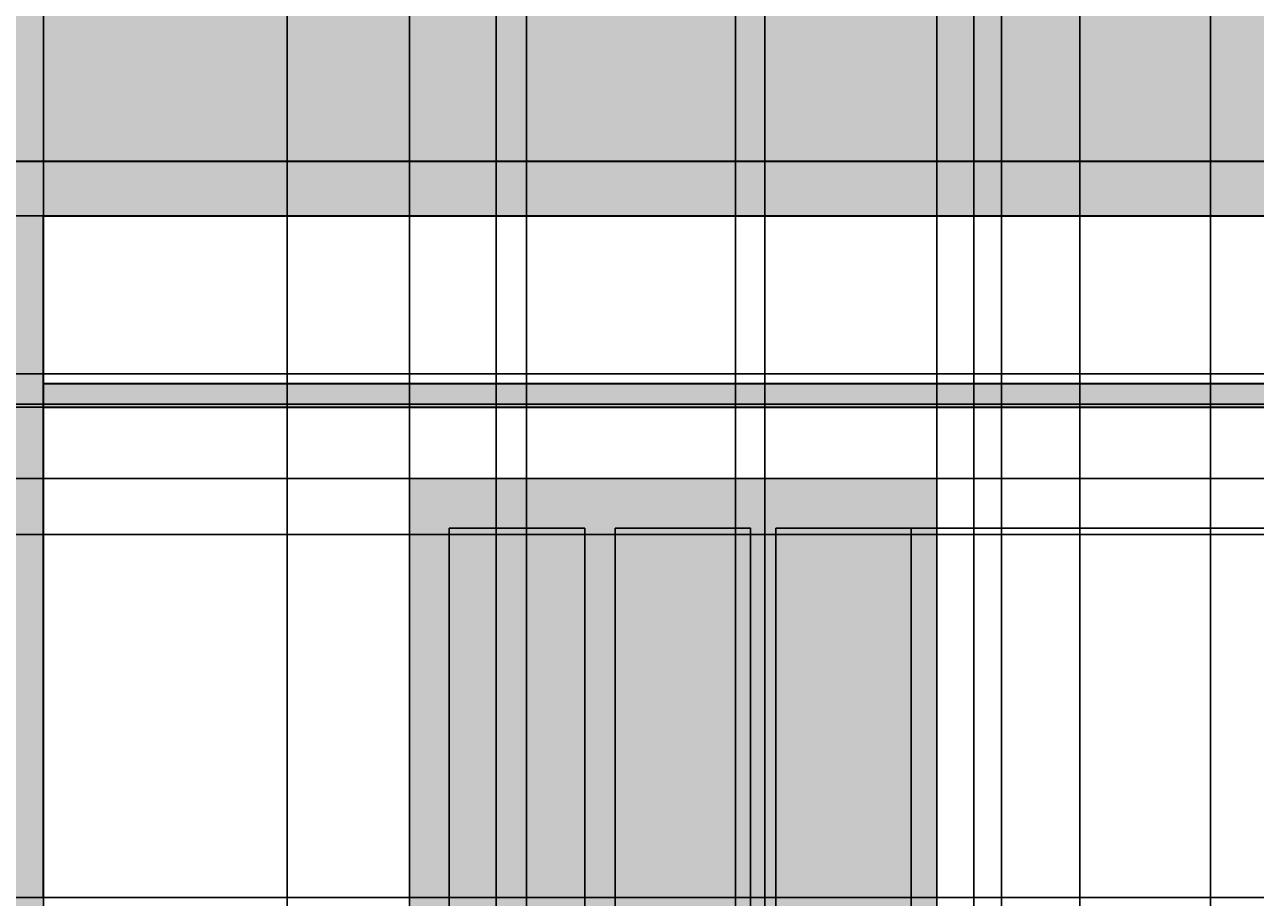
# Model space of a CAD drawing. Units: inches. Extents: x -5 to 714, y 84 to 644.
# Tile 6 of 20: x 266 to 457, y 201 to 336. Entities that reach past the tile are written whole.
import ezdxf

# ---------------------------------------------------------------- set-up
doc = ezdxf.new("R2010")
doc.units = ezdxf.units.IN
doc.header["$MEASUREMENT"] = 0
for name, color, linetype, lineweight in [('A-ANNO-DIMS', 2, 'Continuous', 18), ('A-ELEV', 7, 'Continuous', 35), ('A-ELEV-PATT', 8, 'Continuous', 13), ('A-GLAZ', 3, 'Continuous', 25)]:
    doc.layers.add(name, color=color, linetype=linetype, lineweight=lineweight)
doc.styles.get("Standard").update_dxf_attribs({"font": 'arial.ttf'})
doc.dimstyles.get("Standard").update_dxf_attribs({"dimtxt": 0.9375, "dimasz": 0.18, "dimexe": 0.18, "dimexo": 0.0625, "dimgap": 0.09, "dimtad": 0, "dimtih": 1, "dimtoh": 1, "dimdec": 4, "dimzin": 0, "dimdsep": 46, "dimlunit": 4, "dimtxsty": 'Standard', "dimcen": 0.09, "dimadec": 0, "dimazin": 0, "dimtfac": 1, "dimtdec": 4, "dimtofl": 0, "dimtmove": 0, "dimatfit": 3, "dimfxl": 1, "dimtolj": 1, "dimtzin": 0, "dimarcsym": 0})

# ---------------------------------------------------------------- blocks, each defined once
blk = doc.blocks.new('*D29')
at = {"layer": 'A-ANNO-DIMS', "color": 0, "lineweight": -2, "transparency": 16777216}
for p, q in [((135.73, 471.11), (135.73, 84.31)), ((429.51, 471.11), (429.51, 84.31)), ((135.91, 84.49), (280.94, 84.49)), ((429.33, 84.49), (284.3, 84.49))]:
    blk.add_line(p, q, dxfattribs=at)
at = {"layer": 'A-ANNO-DIMS', "color": 0, "transparency": 16777216}
for points in [[(135.91, 84.52), (135.91, 84.46), (135.73, 84.49)], [(429.33, 84.52), (429.33, 84.46), (429.51, 84.49)]]:
    blk.add_solid(points, dxfattribs=at)
at = {"layer": 'Defpoints', "color": 0, "transparency": 16777216}
for p in [(135.73, 471.17), (429.51, 471.17), (429.51, 84.49)]:
    blk.add_point(p, dxfattribs=at)
at = {"layer": 'A-ANNO-DIMS', "color": 0, "transparency": 16777216, "insert": (282.62, 84.49), "char_height": 0.938, "attachment_point": 5}
blk.add_mtext('\\A1;293.8', dxfattribs=at)
blk = doc.blocks.new('*D53')
at = {"layer": 'A-ANNO-DIMS', "color": 0, "lineweight": -2, "transparency": 16777216}
for p, q in [((259.07, 315.03), (259.07, 84.31)), ((269.24, 306.57), (269.24, 84.31)), ((259.25, 84.49), (262.16, 84.49)), ((269.06, 84.49), (266.15, 84.49))]:
    blk.add_line(p, q, dxfattribs=at)
at = {"layer": 'A-ANNO-DIMS', "color": 0, "transparency": 16777216}
for points in [[(259.25, 84.52), (259.25, 84.46), (259.07, 84.49)], [(269.06, 84.52), (269.06, 84.46), (269.24, 84.49)]]:
    blk.add_solid(points, dxfattribs=at)
at = {"layer": 'Defpoints', "color": 0, "transparency": 16777216}
for p in [(259.07, 315.1), (269.24, 306.63), (269.24, 84.49)]:
    blk.add_point(p, dxfattribs=at)
at = {"layer": 'A-ANNO-DIMS', "color": 0, "transparency": 16777216, "insert": (264.16, 84.49), "char_height": 0.938, "attachment_point": 5}
blk.add_mtext('\\A1;10.178', dxfattribs=at)
blk = doc.blocks.new('*D54')
at = {"layer": 'A-ANNO-DIMS', "color": 0, "lineweight": -2, "transparency": 16777216}
for p, q in [((259.07, 315.16), (259.07, 643.61)), ((259.25, 643.43), (424.21, 643.43)), ((593.25, 643.43), (428.28, 643.43)), ((593.43, 315.16), (593.43, 643.61))]:
    blk.add_line(p, q, dxfattribs=at)
at = {"layer": 'A-ANNO-DIMS', "color": 0, "transparency": 16777216}
for points in [[(259.25, 643.46), (259.25, 643.4), (259.07, 643.43)], [(593.25, 643.46), (593.25, 643.4), (593.43, 643.43)]]:
    blk.add_solid(points, dxfattribs=at)
at = {"layer": 'Defpoints', "color": 0, "transparency": 16777216}
for p in [(593.43, 643.43), (259.07, 315.1), (593.43, 315.1)]:
    blk.add_point(p, dxfattribs=at)
at = {"layer": 'A-ANNO-DIMS', "color": 0, "transparency": 16777216, "insert": (426.25, 643.43), "char_height": 0.938, "attachment_point": 5}
blk.add_mtext('\\A1;334.36', dxfattribs=at)
blk = doc.blocks.new('*D56')
at = {"layer": 'A-ANNO-DIMS', "color": 0, "lineweight": -2, "transparency": 16777216}
for p, q in [((578.03, 277.05), (-2.74, 277.05)), ((-2.56, 276.87), (-2.56, 239.69)), ((-2.56, 201.37), (-2.56, 238.55)), ((578.03, 201.19), (-2.74, 201.19))]:
    blk.add_line(p, q, dxfattribs=at)
at = {"layer": 'A-ANNO-DIMS', "color": 0, "transparency": 16777216}
for points in [[(-2.59, 276.87), (-2.53, 276.87), (-2.56, 277.05)], [(-2.59, 201.37), (-2.53, 201.37), (-2.56, 201.19)]]:
    blk.add_solid(points, dxfattribs=at)
at = {"layer": 'Defpoints', "color": 0, "transparency": 16777216}
for p in [(-2.56, 277.05), (578.09, 277.05), (578.09, 201.19)]:
    blk.add_point(p, dxfattribs=at)
at = {"layer": 'A-ANNO-DIMS', "color": 0, "transparency": 16777216, "insert": (-2.56, 239.12), "char_height": 0.938, "attachment_point": 5}
blk.add_mtext('\\A1;75.86', dxfattribs=at)
blk = doc.blocks.new('*D57')
at = {"layer": 'A-ANNO-DIMS', "color": 0, "lineweight": -2, "transparency": 16777216}
for p, q in [((578.03, 306.63), (-2.74, 306.63)), ((-2.56, 306.45), (-2.56, 292.41)), ((-2.56, 277.23), (-2.56, 291.27)), ((578.03, 277.05), (-2.74, 277.05))]:
    blk.add_line(p, q, dxfattribs=at)
at = {"layer": 'A-ANNO-DIMS', "color": 0, "transparency": 16777216}
for points in [[(-2.59, 306.45), (-2.53, 306.45), (-2.56, 306.63)], [(-2.59, 277.23), (-2.53, 277.23), (-2.56, 277.05)]]:
    blk.add_solid(points, dxfattribs=at)
at = {"layer": 'Defpoints', "color": 0, "transparency": 16777216}
for p in [(578.09, 306.63), (-2.56, 277.05), (578.09, 277.05)]:
    blk.add_point(p, dxfattribs=at)
at = {"layer": 'A-ANNO-DIMS', "color": 0, "transparency": 16777216, "insert": (-2.56, 291.84), "char_height": 0.938, "attachment_point": 5}
blk.add_mtext('\\A1;29.58', dxfattribs=at)
blk = doc.blocks.new('*D59')
at = {"layer": 'A-ANNO-DIMS', "color": 0, "lineweight": -2, "transparency": 16777216}
for p, q in [((593.37, 282.2), (-2.74, 282.2)), ((-2.56, 282.02), (-2.56, 280.41)), ((-2.56, 277.66), (-2.56, 279.27)), ((593.37, 277.48), (-2.74, 277.48))]:
    blk.add_line(p, q, dxfattribs=at)
at = {"layer": 'A-ANNO-DIMS', "color": 0, "transparency": 16777216}
for points in [[(-2.59, 282.02), (-2.53, 282.02), (-2.56, 282.2)], [(-2.59, 277.66), (-2.53, 277.66), (-2.56, 277.48)]]:
    blk.add_solid(points, dxfattribs=at)
at = {"layer": 'Defpoints', "color": 0, "transparency": 16777216}
for p in [(-2.56, 282.2), (593.43, 282.2), (593.43, 277.48)]:
    blk.add_point(p, dxfattribs=at)
at = {"layer": 'A-ANNO-DIMS', "color": 0, "transparency": 16777216, "insert": (-2.56, 279.84), "char_height": 0.938, "attachment_point": 5}
blk.add_mtext('\\A1;4.719', dxfattribs=at)
blk = doc.blocks.new('*D60')
at = {"layer": 'A-ANNO-DIMS', "color": 0, "lineweight": -2, "transparency": 16777216}
for p, q in [((269.24, 277.11), (269.24, 643.61)), ((269.42, 643.43), (295.86, 643.43)), ((325.65, 643.43), (299.21, 643.43)), ((325.83, 266.06), (325.83, 643.61))]:
    blk.add_line(p, q, dxfattribs=at)
at = {"layer": 'A-ANNO-DIMS', "color": 0, "transparency": 16777216}
for points in [[(269.42, 643.46), (269.42, 643.4), (269.24, 643.43)], [(325.65, 643.46), (325.65, 643.4), (325.83, 643.43)]]:
    blk.add_solid(points, dxfattribs=at)
at = {"layer": 'Defpoints', "color": 0, "transparency": 16777216}
for p in [(325.83, 643.43), (269.24, 277.05), (325.83, 266)]:
    blk.add_point(p, dxfattribs=at)
at = {"layer": 'A-ANNO-DIMS', "color": 0, "transparency": 16777216, "insert": (297.54, 643.43), "char_height": 0.938, "attachment_point": 5}
blk.add_mtext('\\A1;56.59', dxfattribs=at)
blk = doc.blocks.new('*D61')
at = {"layer": 'A-ANNO-DIMS', "color": 0, "lineweight": -2, "transparency": 16777216}
for p, q in [((325.83, 266.06), (325.83, 643.61)), ((326.01, 643.43), (364.93, 643.43)), ((407.2, 643.43), (368.28, 643.43)), ((407.38, 266.06), (407.38, 643.61))]:
    blk.add_line(p, q, dxfattribs=at)
at = {"layer": 'A-ANNO-DIMS', "color": 0, "transparency": 16777216}
for points in [[(326.01, 643.46), (326.01, 643.4), (325.83, 643.43)], [(407.2, 643.46), (407.2, 643.4), (407.38, 643.43)]]:
    blk.add_solid(points, dxfattribs=at)
at = {"layer": 'Defpoints', "color": 0, "transparency": 16777216}
for p in [(407.38, 643.43), (325.83, 266), (407.38, 266)]:
    blk.add_point(p, dxfattribs=at)
at = {"layer": 'A-ANNO-DIMS', "color": 0, "transparency": 16777216, "insert": (366.61, 643.43), "char_height": 0.938, "attachment_point": 5}
blk.add_mtext('\\A1;81.55', dxfattribs=at)
blk = doc.blocks.new('*D62')
at = {"layer": 'A-ANNO-DIMS', "color": 0, "lineweight": -2, "transparency": 16777216}
for p, q in [((407.38, 266.06), (407.38, 643.61)), ((407.56, 643.43), (449.27, 643.43)), ((493.6, 643.43), (451.89, 643.43)), ((493.78, 266.06), (493.78, 643.61))]:
    blk.add_line(p, q, dxfattribs=at)
at = {"layer": 'A-ANNO-DIMS', "color": 0, "transparency": 16777216}
for points in [[(407.56, 643.46), (407.56, 643.4), (407.38, 643.43)], [(493.6, 643.46), (493.6, 643.4), (493.78, 643.43)]]:
    blk.add_solid(points, dxfattribs=at)
at = {"layer": 'Defpoints', "color": 0, "transparency": 16777216}
for p in [(493.78, 643.43), (407.38, 266), (493.78, 266)]:
    blk.add_point(p, dxfattribs=at)
at = {"layer": 'A-ANNO-DIMS', "color": 0, "transparency": 16777216, "insert": (450.58, 643.43), "char_height": 0.938, "attachment_point": 5}
blk.add_mtext('\\A1;86.4', dxfattribs=at)
blk = doc.blocks.new('*D65')
at = {"layer": 'A-ANNO-DIMS', "color": 0, "lineweight": -2, "transparency": 16777216}
for p, q in [((325.77, 266), (-2.74, 266)), ((-2.56, 265.82), (-2.56, 219.13)), ((-2.56, 171.3), (-2.56, 217.99)), ((325.77, 171.12), (-2.74, 171.12))]:
    blk.add_line(p, q, dxfattribs=at)
at = {"layer": 'A-ANNO-DIMS', "color": 0, "transparency": 16777216}
for points in [[(-2.59, 265.82), (-2.53, 265.82), (-2.56, 266)], [(-2.59, 171.3), (-2.53, 171.3), (-2.56, 171.12)]]:
    blk.add_solid(points, dxfattribs=at)
at = {"layer": 'Defpoints', "color": 0, "transparency": 16777216}
for p in [(-2.56, 266), (325.83, 266), (325.83, 171.12)]:
    blk.add_point(p, dxfattribs=at)
at = {"layer": 'A-ANNO-DIMS', "color": 0, "transparency": 16777216, "insert": (-2.56, 218.56), "char_height": 0.938, "attachment_point": 5}
blk.add_mtext('\\A1;94.88', dxfattribs=at)
blk = doc.blocks.new('*D66')
at = {"layer": 'A-ANNO-DIMS', "color": 0, "lineweight": -2, "transparency": 16777216}
for p, q in [((332.01, 258.22), (332.01, 84.31)), ((352.95, 258.22), (352.95, 84.31)), ((332.19, 84.49), (340.43, 84.49)), ((352.77, 84.49), (344.52, 84.49))]:
    blk.add_line(p, q, dxfattribs=at)
at = {"layer": 'A-ANNO-DIMS', "color": 0, "transparency": 16777216}
for points in [[(332.19, 84.52), (332.19, 84.46), (332.01, 84.49)], [(352.77, 84.52), (352.77, 84.46), (352.95, 84.49)]]:
    blk.add_solid(points, dxfattribs=at)
at = {"layer": 'Defpoints', "color": 0, "transparency": 16777216}
for p in [(332.01, 258.29), (352.95, 258.29), (352.95, 84.49)]:
    blk.add_point(p, dxfattribs=at)
at = {"layer": 'A-ANNO-DIMS', "color": 0, "transparency": 16777216, "insert": (342.48, 84.49), "char_height": 0.938, "attachment_point": 5}
blk.add_mtext('\\A1;20.943', dxfattribs=at)
blk = doc.blocks.new('*D67')
at = {"layer": 'A-ANNO-DIMS', "color": 0, "lineweight": -2, "transparency": 16777216}
for p, q in [((357.65, 258.22), (357.65, 84.31)), ((378.6, 258.22), (378.6, 84.31)), ((357.83, 84.49), (366.08, 84.49)), ((378.42, 84.49), (370.17, 84.49))]:
    blk.add_line(p, q, dxfattribs=at)
at = {"layer": 'A-ANNO-DIMS', "color": 0, "transparency": 16777216}
for points in [[(357.83, 84.52), (357.83, 84.46), (357.65, 84.49)], [(378.42, 84.52), (378.42, 84.46), (378.6, 84.49)]]:
    blk.add_solid(points, dxfattribs=at)
at = {"layer": 'Defpoints', "color": 0, "transparency": 16777216}
for p in [(357.65, 258.29), (378.6, 258.29), (378.6, 84.49)]:
    blk.add_point(p, dxfattribs=at)
at = {"layer": 'A-ANNO-DIMS', "color": 0, "transparency": 16777216, "insert": (368.12, 84.49), "char_height": 0.938, "attachment_point": 5}
blk.add_mtext('\\A1;20.943', dxfattribs=at)
blk = doc.blocks.new('*D68')
at = {"layer": 'A-ANNO-DIMS', "color": 0, "lineweight": -2, "transparency": 16777216}
for p, q in [((382.5, 258.22), (382.5, 84.31)), ((403.44, 258.22), (403.44, 84.31)), ((382.68, 84.49), (390.92, 84.49)), ((403.26, 84.49), (395.01, 84.49))]:
    blk.add_line(p, q, dxfattribs=at)
at = {"layer": 'A-ANNO-DIMS', "color": 0, "transparency": 16777216}
for points in [[(382.68, 84.52), (382.68, 84.46), (382.5, 84.49)], [(403.26, 84.52), (403.26, 84.46), (403.44, 84.49)]]:
    blk.add_solid(points, dxfattribs=at)
at = {"layer": 'Defpoints', "color": 0, "transparency": 16777216}
for p in [(382.5, 258.29), (403.44, 258.29), (403.44, 84.49)]:
    blk.add_point(p, dxfattribs=at)
at = {"layer": 'A-ANNO-DIMS', "color": 0, "transparency": 16777216, "insert": (392.97, 84.49), "char_height": 0.938, "attachment_point": 5}
blk.add_mtext('\\A1;20.943', dxfattribs=at)
blk = doc.blocks.new('*D69')
at = {"layer": 'A-ANNO-DIMS', "color": 0, "lineweight": -2, "transparency": 16777216}
for p, q in [((403.5, 258.29), (712.66, 258.29)), ((712.48, 258.11), (712.48, 216.52)), ((712.48, 173.8), (712.48, 215.38)), ((403.5, 173.62), (712.66, 173.62))]:
    blk.add_line(p, q, dxfattribs=at)
at = {"layer": 'A-ANNO-DIMS', "color": 0, "transparency": 16777216}
for points in [[(712.45, 258.11), (712.51, 258.11), (712.48, 258.29)], [(712.45, 173.8), (712.51, 173.8), (712.48, 173.62)]]:
    blk.add_solid(points, dxfattribs=at)
at = {"layer": 'Defpoints', "color": 0, "transparency": 16777216}
for p in [(403.44, 258.29), (712.48, 258.29), (403.44, 173.62)]:
    blk.add_point(p, dxfattribs=at)
at = {"layer": 'A-ANNO-DIMS', "color": 0, "transparency": 16777216, "insert": (712.48, 215.95), "char_height": 0.938, "attachment_point": 5}
blk.add_mtext('\\A1;84.67', dxfattribs=at)
blk = doc.blocks.new('*D71')
at = {"layer": 'A-ANNO-DIMS', "color": 0, "lineweight": -2, "transparency": 16777216}
for p, q in [((537.12, 257.34), (-2.74, 257.34)), ((-2.56, 257.16), (-2.56, 229.83)), ((-2.56, 201.37), (-2.56, 228.7)), ((537.12, 201.19), (-2.74, 201.19))]:
    blk.add_line(p, q, dxfattribs=at)
at = {"layer": 'A-ANNO-DIMS', "color": 0, "transparency": 16777216}
for points in [[(-2.59, 257.16), (-2.53, 257.16), (-2.56, 257.34)], [(-2.59, 201.37), (-2.53, 201.37), (-2.56, 201.19)]]:
    blk.add_solid(points, dxfattribs=at)
at = {"layer": 'Defpoints', "color": 0, "transparency": 16777216}
for p in [(-2.56, 257.34), (537.18, 257.34), (537.18, 201.19)]:
    blk.add_point(p, dxfattribs=at)
at = {"layer": 'A-ANNO-DIMS', "color": 0, "transparency": 16777216, "insert": (-2.56, 229.27), "char_height": 0.938, "attachment_point": 5}
blk.add_mtext('\\A1;56.15', dxfattribs=at)
blk = doc.blocks.new('*D72')
at = {"layer": 'A-ANNO-DIMS', "color": 0, "lineweight": -2, "transparency": 16777216}
for p, q in [((493.71, 266), (-2.74, 266)), ((-2.56, 265.82), (-2.56, 234.17)), ((-2.56, 201.37), (-2.56, 233.03)), ((493.71, 201.19), (-2.74, 201.19))]:
    blk.add_line(p, q, dxfattribs=at)
at = {"layer": 'A-ANNO-DIMS', "color": 0, "transparency": 16777216}
for points in [[(-2.59, 265.82), (-2.53, 265.82), (-2.56, 266)], [(-2.59, 201.37), (-2.53, 201.37), (-2.56, 201.19)]]:
    blk.add_solid(points, dxfattribs=at)
at = {"layer": 'Defpoints', "color": 0, "transparency": 16777216}
for p in [(-2.56, 266), (493.78, 266), (493.78, 201.19)]:
    blk.add_point(p, dxfattribs=at)
at = {"layer": 'A-ANNO-DIMS', "color": 0, "transparency": 16777216, "insert": (-2.56, 233.6), "char_height": 0.938, "attachment_point": 5}
blk.add_mtext('\\A1;64.81', dxfattribs=at)
blk = doc.blocks.new('*D83')
at = {"layer": 'A-ANNO-DIMS', "color": 0, "lineweight": -2, "transparency": 16777216}
for p, q in [((306.96, 144.93), (306.96, 643.61)), ((307.14, 643.43), (321.53, 643.43)), ((339.09, 643.43), (324.69, 643.43)), ((339.27, 144.93), (339.27, 643.61))]:
    blk.add_line(p, q, dxfattribs=at)
at = {"layer": 'A-ANNO-DIMS', "color": 0, "transparency": 16777216}
for points in [[(307.14, 643.46), (307.14, 643.4), (306.96, 643.43)], [(339.09, 643.46), (339.09, 643.4), (339.27, 643.43)]]:
    blk.add_solid(points, dxfattribs=at)
at = {"layer": 'Defpoints', "color": 0, "transparency": 16777216}
for p in [(339.27, 643.43), (306.96, 144.86), (339.27, 144.86)]:
    blk.add_point(p, dxfattribs=at)
at = {"layer": 'A-ANNO-DIMS', "color": 0, "transparency": 16777216, "insert": (323.11, 643.43), "char_height": 0.938, "attachment_point": 5}
blk.add_mtext('\\A1;32.31', dxfattribs=at)
blk = doc.blocks.new('*D84')
at = {"layer": 'A-ANNO-DIMS', "color": 0, "lineweight": -2, "transparency": 16777216}
for p, q in [((343.97, 144.93), (343.97, 643.61)), ((344.15, 643.43), (358.54, 643.43)), ((376.1, 643.43), (361.71, 643.43)), ((376.28, 144.93), (376.28, 643.61))]:
    blk.add_line(p, q, dxfattribs=at)
at = {"layer": 'A-ANNO-DIMS', "color": 0, "transparency": 16777216}
for points in [[(344.15, 643.46), (344.15, 643.4), (343.97, 643.43)], [(376.1, 643.46), (376.1, 643.4), (376.28, 643.43)]]:
    blk.add_solid(points, dxfattribs=at)
at = {"layer": 'Defpoints', "color": 0, "transparency": 16777216}
for p in [(376.28, 643.43), (343.97, 144.86), (376.28, 144.86)]:
    blk.add_point(p, dxfattribs=at)
at = {"layer": 'A-ANNO-DIMS', "color": 0, "transparency": 16777216, "insert": (360.13, 643.43), "char_height": 0.938, "attachment_point": 5}
blk.add_mtext('\\A1;32.31', dxfattribs=at)
blk = doc.blocks.new('*D85')
at = {"layer": 'A-ANNO-DIMS', "color": 0, "lineweight": -2, "transparency": 16777216}
for p, q in [((380.78, 144.93), (380.78, 643.61)), ((380.96, 643.43), (395.35, 643.43)), ((412.91, 643.43), (398.51, 643.43)), ((413.09, 144.93), (413.09, 643.61))]:
    blk.add_line(p, q, dxfattribs=at)
at = {"layer": 'A-ANNO-DIMS', "color": 0, "transparency": 16777216}
for points in [[(380.96, 643.46), (380.96, 643.4), (380.78, 643.43)], [(412.91, 643.46), (412.91, 643.4), (413.09, 643.43)]]:
    blk.add_solid(points, dxfattribs=at)
at = {"layer": 'Defpoints', "color": 0, "transparency": 16777216}
for p in [(413.09, 643.43), (380.78, 144.86), (413.09, 144.86)]:
    blk.add_point(p, dxfattribs=at)
at = {"layer": 'A-ANNO-DIMS', "color": 0, "transparency": 16777216, "insert": (396.93, 643.43), "char_height": 0.938, "attachment_point": 5}
blk.add_mtext('\\A1;32.31', dxfattribs=at)
blk = doc.blocks.new('*D86')
at = {"layer": 'A-ANNO-DIMS', "color": 0, "lineweight": -2, "transparency": 16777216}
for p, q in [((417.38, 144.93), (417.38, 643.61)), ((417.56, 643.43), (431.96, 643.43)), ((449.51, 643.43), (435.12, 643.43)), ((449.69, 144.93), (449.69, 643.61))]:
    blk.add_line(p, q, dxfattribs=at)
at = {"layer": 'A-ANNO-DIMS', "color": 0, "transparency": 16777216}
for points in [[(417.56, 643.46), (417.56, 643.4), (417.38, 643.43)], [(449.51, 643.46), (449.51, 643.4), (449.69, 643.43)]]:
    blk.add_solid(points, dxfattribs=at)
at = {"layer": 'Defpoints', "color": 0, "transparency": 16777216}
for p in [(449.69, 643.43), (417.38, 144.86), (449.69, 144.86)]:
    blk.add_point(p, dxfattribs=at)
at = {"layer": 'A-ANNO-DIMS', "color": 0, "transparency": 16777216, "insert": (433.54, 643.43), "char_height": 0.938, "attachment_point": 5}
blk.add_mtext('\\A1;32.31', dxfattribs=at)

msp = doc.modelspace()

# ---------------------------------------------------------------- hatches: boundary and pattern name
at = {"layer": 'A-ELEV-PATT', "transparency": 33554687}
h = msp.add_hatch(color=256, dxfattribs=at)
h.dxf.hatch_style = 1
h.paths.add_polyline_path([(188.3677, 525.1928), (67.9893, 525.1928), (67.9893, 489.1928), (67.9893, 345.1928), (126.7303, 345.1928), (126.7303, 480.1709), (229.3575, 480.1709), (229.3575, 525.1928), (212.6043, 525.1928), (212.6043, 482.7164), (211.0019, 482.7164), (211.0019, 525.1928), (207.6919, 525.1928), (199.9852, 525.1928), (199.9852, 482.7164), (198.3828, 482.7164), (198.3828, 525.1928), (189.9701, 525.1928), (189.9701, 482.7164), (188.3677, 482.7164)])
h.paths.add_polyline_path([(121.3589, 336.2066), (75.5048, 336.2066), (75.5048, 319.345), (121.3589, 319.345)])
h.paths.add_polyline_path([(121.3589, 319.345), (75.5048, 319.345), (75.5048, 302.3045), (121.3589, 302.3045)])
h.paths.add_polyline_path([(121.3589, 302.3045), (75.5048, 302.3045), (75.5048, 282.8561), (121.3589, 282.8561)])
h.paths.add_polyline_path([(121.3589, 282.8561), (75.5048, 282.8561), (75.5048, 261.5556), (121.3589, 261.5556)])
h.paths.add_polyline_path([(121.3589, 261.5556), (75.5048, 261.5556), (75.5048, 243.7009), (121.3589, 243.7009)])
h.paths.add_polyline_path([(121.3589, 243.7009), (75.5048, 243.7009), (75.5048, 223.5117), (121.3589, 223.5117)])
h.paths.add_polyline_path([(121.3589, 223.5117), (75.5048, 223.5117), (75.5048, 212.5836), (121.3589, 212.5836)])
h.paths.add_polyline_path([(121.3589, 212.5836), (75.5048, 212.5836), (75.5048, 201.1928), (121.3589, 201.1928)])
h.paths.add_polyline_path([(179.9335, 201.1928), (30.1395, 201.1928), (30.1395, 198.7054), (179.9335, 198.7054)])
h.paths.add_polyline_path([(187.6349, 201.1928), (179.9335, 201.1928), (179.9335, 198.7054), (179.9335, 141.1928), (269.2446, 141.1928), (269.2446, 201.1928), (263.4349, 201.1928), (263.4349, 152.1176), (187.6349, 152.1176)])
h.paths.add_polyline_path([(269.2446, 277.0513), (269.2446, 287.501), (269.2446, 306.6286), (578.0915, 306.6286), (578.0915, 201.1928), (593.428, 201.1928), (593.428, 315.0968), (584.4202, 315.0968), (259.0665, 315.0968), (259.0665, 201.1928), (263.4349, 201.1928), (269.2446, 201.1928)])
h = msp.add_hatch(color=256, dxfattribs=at)
h.dxf.hatch_style = 1
h.paths.add_polyline_path([(584.2229, 343.1928), (259.0665, 343.1928), (259.0665, 315.0968), (584.2229, 315.0968)])
h.paths.add_polyline_path([(352.9482, 258.2864), (332.0052, 258.2864), (332.0052, 201.1928), (352.9482, 201.1928)])
h.paths.add_polyline_path([(378.5957, 258.2864), (357.6527, 258.2864), (357.6527, 201.1928), (378.5957, 201.1928)])
h.paths.add_polyline_path([(403.4391, 258.2864), (382.4961, 258.2864), (382.4961, 201.1928), (403.4391, 201.1928)])
h.paths.add_polyline_path([(339.2672, 197.3754), (332.0052, 197.3754), (332.0052, 191.3028), (339.2672, 191.3028)])
h.paths.add_polyline_path([(352.9482, 197.3754), (343.9704, 197.3754), (343.9704, 191.3028), (352.9482, 191.3028)])
h.paths.add_polyline_path([(352.9482, 189.3028), (343.9704, 189.3028), (343.9704, 184.8307), (352.9482, 184.8307)])
h.paths.add_polyline_path([(339.2672, 189.3028), (332.0052, 189.3028), (332.0052, 184.8307), (339.2672, 184.8307)])
h.paths.add_polyline_path([(339.2672, 182.8307), (332.0052, 182.8307), (332.0052, 177.6504), (339.2672, 177.6504)])
h.paths.add_polyline_path([(352.9482, 182.8307), (343.9704, 182.8307), (343.9704, 177.6504), (352.9482, 177.6504)])
h.paths.add_polyline_path([(352.9482, 175.6504), (343.9704, 175.6504), (343.9704, 173.6169), (352.9482, 173.6169)])
h.paths.add_polyline_path([(339.2672, 175.6504), (332.0052, 175.6504), (332.0052, 173.6169), (339.2672, 173.6169)])
h.paths.add_polyline_path([(376.2796, 175.6504), (357.6527, 175.6504), (357.6527, 173.6169), (376.2796, 173.6169)])
h.paths.add_polyline_path([(376.2796, 182.8307), (357.6527, 182.8307), (357.6527, 177.6504), (376.2796, 177.6504)])
h.paths.add_polyline_path([(376.2796, 189.3028), (357.6527, 189.3028), (357.6527, 184.8307), (376.2796, 184.8307)])
h.paths.add_polyline_path([(376.2796, 197.3754), (357.6527, 197.3754), (357.6527, 191.3028), (376.2796, 191.3028)])
h.paths.add_polyline_path([(403.4391, 197.3754), (382.4961, 197.3754), (382.4961, 191.3028), (403.4391, 191.3028)])
h.paths.add_polyline_path([(403.4391, 189.3028), (382.4961, 189.3028), (382.4961, 184.8307), (403.4391, 184.8307)])
h.paths.add_polyline_path([(403.4391, 182.8307), (382.4961, 182.8307), (382.4961, 177.6504), (403.4391, 177.6504)])
h.paths.add_polyline_path([(403.4391, 175.6504), (382.4961, 175.6504), (382.4961, 173.6169), (403.4391, 173.6169)])
h = msp.add_hatch(color=256, dxfattribs=at)
h.dxf.hatch_style = 1
h.paths.add_polyline_path([(578.0915, 280.7123), (269.2446, 280.7123), (269.2446, 277.0513), (578.0915, 277.0513)])
h = msp.add_hatch(color=256, dxfattribs=at)
h.dxf.hatch_style = 1
h.paths.add_polyline_path([(407.3813, 266.0021), (325.8305, 266.0021), (325.8305, 201.1928), (332.0052, 201.1928), (332.0052, 258.2864), (352.9482, 258.2864), (352.9482, 201.1928), (357.6527, 201.1928), (357.6527, 258.2864), (378.5957, 258.2864), (378.5957, 201.1928), (382.4961, 201.1928), (382.4961, 258.2864), (403.4391, 258.2864), (403.4391, 201.1928), (407.3813, 201.1928)])
h = msp.add_hatch(color=256, dxfattribs=at)
h.dxf.hatch_style = 1
h.paths.add_polyline_path([(449.6911, 151.1385), (417.3818, 151.1385), (417.3818, 149.1385), (449.6911, 149.1385)])
h.paths.add_polyline_path([(449.6911, 157.2254), (417.3818, 157.2254), (417.3818, 155.2254), (449.6911, 155.2254)])
h.paths.add_polyline_path([(449.6911, 163.4201), (417.3818, 163.4201), (417.3818, 161.4201), (449.6911, 161.4201)])
h.paths.add_polyline_path([(449.6911, 170.0006), (417.3818, 170.0006), (417.3818, 168.0006), (449.6911, 168.0006)])
h.paths.add_polyline_path([(449.6911, 177.6504), (417.3818, 177.6504), (417.3818, 175.6504), (449.6911, 175.6504)])
h.paths.add_polyline_path([(449.6911, 184.8307), (417.3818, 184.8307), (417.3818, 182.8307), (449.6911, 182.8307)])
h.paths.add_polyline_path([(449.6911, 191.3028), (417.3818, 191.3028), (417.3818, 189.3028), (449.6911, 189.3028)])
h.paths.add_polyline_path([(407.3813, 191.3028), (403.4391, 191.3028), (403.4391, 189.3028), (407.3813, 189.3028)])
h.paths.add_polyline_path([(413.0876, 191.3028), (407.3813, 191.3028), (407.3813, 189.3028), (413.0876, 189.3028)])
h.paths.add_polyline_path([(403.4391, 191.3028), (382.4961, 191.3028), (382.4961, 189.3028), (403.4391, 189.3028)])
h.paths.add_polyline_path([(403.4391, 184.8307), (382.4961, 184.8307), (382.4961, 182.8307), (403.4391, 182.8307)])
h.paths.add_polyline_path([(403.4391, 177.6504), (382.4961, 177.6504), (382.4961, 175.6504), (403.4391, 175.6504)])
h.paths.add_polyline_path([(382.4961, 177.6504), (380.7784, 177.6504), (380.7784, 175.6504), (382.4961, 175.6504)], flags=17)
h.paths.add_polyline_path([(343.9704, 173.6169), (339.2672, 173.6169), (339.2672, 171.1197), (343.9704, 171.1197)])
h.paths.add_polyline_path([(343.9704, 197.3754), (352.9482, 197.3754), (352.9482, 258.2864), (332.0052, 258.2864), (332.0052, 197.3754), (339.2672, 197.3754), (339.2672, 173.6169), (343.9704, 173.6169)])
h.paths.add_polyline_path([(339.2672, 191.3028), (332.0052, 191.3028), (332.0052, 189.3028), (339.2672, 189.3028)], flags=17)
h.paths.add_polyline_path([(332.0052, 191.3028), (325.8305, 191.3028), (325.8305, 189.3028), (332.0052, 189.3028)])
h.paths.add_polyline_path([(332.0052, 201.1928), (325.8305, 201.1928), (325.8305, 197.3754), (332.0052, 197.3754)])
h.paths.add_polyline_path([(357.6527, 201.1928), (352.9482, 201.1928), (352.9482, 197.3754), (357.6527, 197.3754)])
h.paths.add_polyline_path([(378.5957, 201.1928), (357.6527, 201.1928), (357.6527, 197.3754), (376.2796, 197.3754), (376.2796, 173.6169), (378.5957, 173.6169)])
h.paths.add_polyline_path([(382.4961, 201.1928), (378.5957, 201.1928), (378.5957, 173.6169), (376.2796, 173.6169), (376.2796, 171.1197), (380.7784, 171.1197), (380.7784, 197.3754), (382.4961, 197.3754)])
h.paths.add_polyline_path([(403.4391, 201.1928), (382.4961, 201.1928), (382.4961, 197.3754), (403.4391, 197.3754)])
h.paths.add_polyline_path([(407.3813, 201.1928), (403.4391, 201.1928), (403.4391, 197.3754), (407.3813, 197.3754)])
h.paths.add_polyline_path([(352.9482, 191.3028), (343.9704, 191.3028), (343.9704, 189.3028), (352.9482, 189.3028)], flags=17)
h.paths.add_polyline_path([(376.2796, 191.3028), (357.6527, 191.3028), (357.6527, 189.3028), (376.2796, 189.3028)], flags=17)
h.paths.add_polyline_path([(332.0052, 184.8307), (325.8305, 184.8307), (325.8305, 182.8307), (332.0052, 182.8307)])
h.paths.add_polyline_path([(339.2672, 184.8307), (332.0052, 184.8307), (332.0052, 182.8307), (339.2672, 182.8307)], flags=17)
h.paths.add_polyline_path([(352.9482, 184.8307), (343.9704, 184.8307), (343.9704, 182.8307), (352.9482, 182.8307)], flags=17)
h.paths.add_polyline_path([(357.6527, 191.3028), (352.9482, 191.3028), (352.9482, 189.3028), (357.6527, 189.3028)])
h.paths.add_polyline_path([(357.6527, 184.8307), (352.9482, 184.8307), (352.9482, 182.8307), (357.6527, 182.8307)])
h.paths.add_polyline_path([(376.2796, 184.8307), (357.6527, 184.8307), (357.6527, 182.8307), (376.2796, 182.8307)], flags=17)
h.paths.add_polyline_path([(357.6527, 177.6504), (352.9482, 177.6504), (352.9482, 175.6504), (357.6527, 175.6504)])
h.paths.add_polyline_path([(376.2796, 177.6504), (357.6527, 177.6504), (357.6527, 175.6504), (376.2796, 175.6504)], flags=17)
h.paths.add_polyline_path([(352.9482, 177.6504), (343.9704, 177.6504), (343.9704, 175.6504), (352.9482, 175.6504)], flags=17)
h.paths.add_polyline_path([(339.2672, 177.6504), (332.0052, 177.6504), (332.0052, 175.6504), (339.2672, 175.6504)], flags=17)
h.paths.add_polyline_path([(332.0052, 177.6504), (325.8305, 177.6504), (325.8305, 175.6504), (332.0052, 175.6504)])
h.paths.add_polyline_path([(382.4961, 191.3028), (380.7784, 191.3028), (380.7784, 189.3028), (382.4961, 189.3028)], flags=17)
h.paths.add_polyline_path([(382.4961, 184.8307), (380.7784, 184.8307), (380.7784, 182.8307), (382.4961, 182.8307)], flags=17)
h.paths.add_polyline_path([(407.3813, 184.8307), (403.4391, 184.8307), (403.4391, 182.8307), (407.3813, 182.8307)])
h.paths.add_polyline_path([(413.0876, 184.8307), (407.3813, 184.8307), (407.3813, 182.8307), (413.0876, 182.8307)])
h.paths.add_polyline_path([(407.3813, 177.6504), (403.4391, 177.6504), (403.4391, 175.6504), (407.3813, 175.6504)])
h.paths.add_polyline_path([(413.0876, 177.6504), (407.3813, 177.6504), (407.3813, 175.6504), (413.0876, 175.6504)])
h = msp.add_hatch(color=256, dxfattribs=at)
h.dxf.hatch_style = 1
h.paths.add_polyline_path([(352.9482, 258.2864), (332.0052, 258.2864), (332.0052, 201.1928), (352.9482, 201.1928)])

# ---------------------------------------------------------------- linework, layer by layer
at = {"layer": 'A-ELEV'}
for p, q in [((259.0665, 315.0968), (584.4202, 315.0968)), ((269.2446, 287.501), (269.2446, 306.6286)), ((269.2446, 306.6286), (578.0915, 306.6286)), ((269.2446, 277.0513), (269.2446, 287.501)), ((269.2446, 280.7123), (578.0915, 280.7123)), ((269.2446, 201.1928), (269.2446, 277.0513)), ((269.2446, 277.0513), (578.0915, 277.0513))]:
    msp.add_line(p, q, dxfattribs=at)
at = {"layer": 'A-GLAZ'}
for points in [[(325.8305, 266.0021), (407.3813, 266.0021), (407.3813, 171.1197), (325.8305, 171.1197)], [(332.0052, 258.2864), (352.9482, 258.2864), (352.9482, 173.6169), (332.0052, 173.6169)], [(357.6527, 258.2864), (378.5957, 258.2864), (378.5957, 173.6169), (357.6527, 173.6169)], [(382.4961, 258.2864), (403.4391, 258.2864), (403.4391, 173.6169), (382.4961, 173.6169)]]:
    msp.add_lwpolyline(points, close=True, dxfattribs=at)

# ---------------------------------------------------------------- dimensions: what is measured, and where the dimension line sits
at = {"layer": 'A-ANNO-DIMS'}
for base, p1, p2, override, picture, middle in [((593.428, 643.4276), (259.0665, 315.0968), (593.428, 315.0968), {"dimdec": 2, "dimlfac": 1, "dimrnd": 0, "dimzin": 0, "dimdsep": 46, "dimlunit": 2}, '*D54', (426.2472, 643.4276)), ((325.8305, 643.4276), (269.2446, 277.0513), (325.8305, 266.0021), {"dimdec": 2, "dimlfac": 1, "dimrnd": 0, "dimzin": 0, "dimdsep": 46, "dimlunit": 2}, '*D60', (297.5375, 643.4276)), ((339.2672, 643.4276), (306.958, 144.8639), (339.2672, 144.8639), {"dimdec": 2, "dimlfac": 1, "dimrnd": 0, "dimzin": 0, "dimdsep": 46, "dimlunit": 2}, '*D83', (323.1126, 643.4276)), ((407.3813, 643.4276), (325.8305, 266.0021), (407.3813, 266.0021), {"dimdec": 2, "dimlfac": 1, "dimrnd": 0, "dimzin": 0, "dimdsep": 46, "dimlunit": 2}, '*D61', (366.6059, 643.4276)), ((376.2796, 643.4276), (343.9704, 144.8639), (376.2796, 144.8639), {"dimdec": 2, "dimlfac": 1, "dimrnd": 0, "dimzin": 0, "dimdsep": 46, "dimlunit": 2}, '*D84', (360.125, 643.4276)), ((413.0876, 643.4276), (380.7784, 144.8639), (413.0876, 144.8639), {"dimdec": 2, "dimlfac": 1, "dimrnd": 0, "dimzin": 0, "dimdsep": 46, "dimlunit": 2}, '*D85', (396.933, 643.4276)), ((493.7771, 643.4276), (407.3813, 266.0021), (493.7771, 266.0021), {"dimdec": 1, "dimlfac": 1, "dimrnd": 0, "dimzin": 0, "dimdsep": 46, "dimlunit": 2}, '*D62', (450.5792, 643.4276)), ((449.6911, 643.4276), (417.3818, 144.8639), (449.6911, 144.8639), {"dimdec": 2, "dimlfac": 1, "dimrnd": 0, "dimzin": 0, "dimdsep": 46, "dimlunit": 2}, '*D86', (433.5365, 643.4276)), ((429.5094, 84.4928), (135.7303, 471.1709), (429.5094, 471.1709), {"dimdec": 1, "dimlfac": 1, "dimrnd": 0, "dimzin": 0, "dimdsep": 46, "dimlunit": 2}, '*D29', (282.6198, 84.4928)), ((269.2446, 84.4928), (259.0665, 315.0968), (269.2446, 306.6286), {"dimdec": 3, "dimlfac": 1, "dimrnd": 0, "dimzin": 0, "dimdsep": 46, "dimlunit": 2}, '*D53', (264.1555, 84.4928)), ((352.9482, 84.4928), (332.0052, 258.2864), (352.9482, 258.2864), {"dimdec": 3, "dimlfac": 1, "dimrnd": 0, "dimzin": 0, "dimdsep": 46, "dimlunit": 2}, '*D66', (342.4767, 84.4928)), ((378.5957, 84.4928), (357.6527, 258.2864), (378.5957, 258.2864), {"dimdec": 3, "dimlfac": 1, "dimrnd": 0, "dimzin": 0, "dimdsep": 46, "dimlunit": 2}, '*D67', (368.1242, 84.4928)), ((403.4391, 84.4928), (382.4961, 258.2864), (403.4391, 258.2864), {"dimdec": 3, "dimlfac": 1, "dimrnd": 0, "dimzin": 0, "dimdsep": 46, "dimlunit": 2}, '*D68', (392.9676, 84.4928))]:
    dim = msp.add_linear_dim(base=base, p1=p1, p2=p2, dimstyle='Standard', override=override, dxfattribs=at)
    dim.commit()
    dim.dimension.update_dxf_attribs({"geometry": picture, "text_midpoint": middle})
for base, p1, p2, override, picture, middle in [((-2.5605, 277.0513), (578.0915, 306.6286), (578.0915, 277.0513), {"dimdec": 2, "dimlfac": 1, "dimrnd": 0, "dimzin": 0, "dimdsep": 46, "dimlunit": 2}, '*D57', (-2.5605, 291.84)), ((-2.5605, 282.1969), (593.428, 277.4776), (593.428, 282.1969), {"dimdec": 3, "dimlfac": 1, "dimrnd": 0, "dimzin": 0, "dimdsep": 46, "dimlunit": 2}, '*D59', (-2.5605, 279.8372)), ((-2.5605, 277.0513), (578.0915, 201.1928), (578.0915, 277.0513), {"dimdec": 2, "dimlfac": 1, "dimrnd": 0, "dimzin": 0, "dimdsep": 46, "dimlunit": 2}, '*D56', (-2.5605, 239.1221)), ((-2.5605, 266.0021), (325.8305, 171.1197), (325.8305, 266.0021), {"dimdec": 2, "dimlfac": 1, "dimrnd": 0, "dimzin": 0, "dimdsep": 46, "dimlunit": 2}, '*D65', (-2.5605, 218.5609)), ((-2.5605, 266.0021), (493.7771, 201.1928), (493.7771, 266.0021), {"dimdec": 2, "dimlfac": 1, "dimrnd": 0, "dimzin": 0, "dimdsep": 46, "dimlunit": 2}, '*D72', (-2.5605, 233.5974)), ((-2.5605, 257.3379), (537.1779, 201.1928), (537.1779, 257.3379), {"dimdec": 2, "dimlfac": 1, "dimrnd": 0, "dimzin": 0, "dimdsep": 46, "dimlunit": 2}, '*D71', (-2.5605, 229.2653)), ((712.4826, 258.2864), (403.4391, 173.6169), (403.4391, 258.2864), {"dimdec": 2, "dimlfac": 1, "dimrnd": 0, "dimzin": 0, "dimdsep": 46, "dimlunit": 2}, '*D69', (712.4826, 215.9517))]:
    dim = msp.add_linear_dim(base=base, p1=p1, p2=p2, angle=90, dimstyle='Standard', override=override, dxfattribs=at)
    dim.commit()
    dim.dimension.update_dxf_attribs({"geometry": picture, "text_midpoint": middle})

doc.saveas('drawing.dxf')
